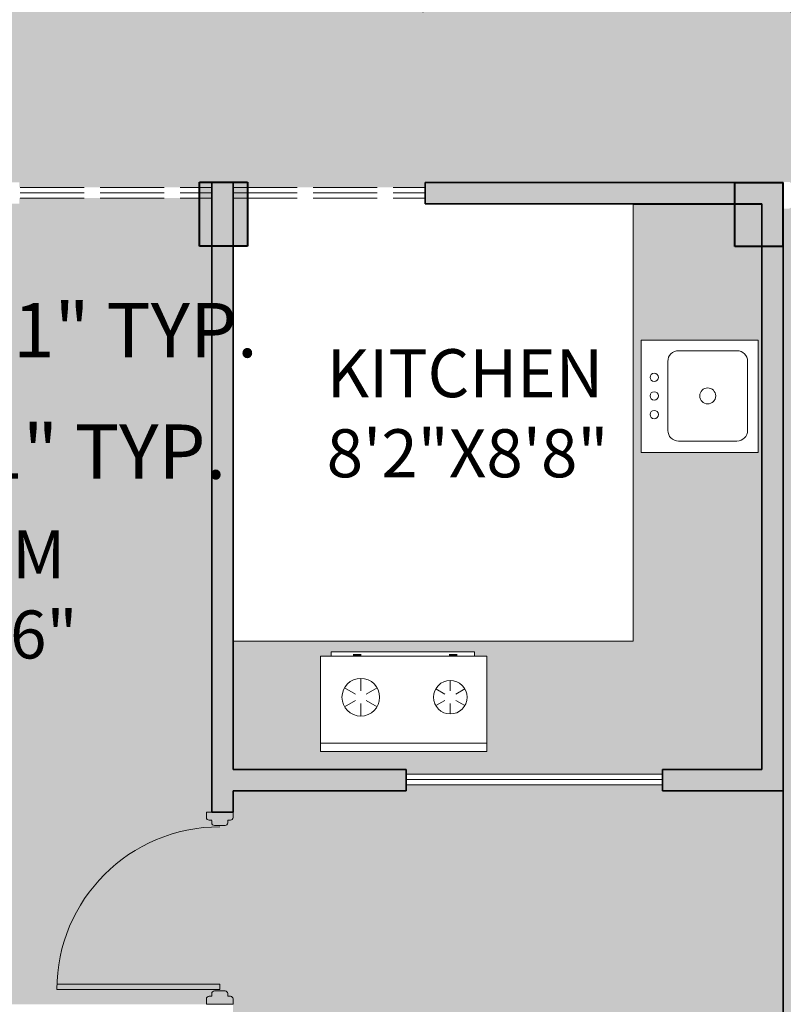
# Model space of a CAD drawing. Units: inches. Extents: x 1077 to 2505, y 1892 to 2728.
# Tile 5 of 26: x 1290 to 1433, y 2153 to 2338. Entities that reach past the tile are written whole.
import ezdxf

# ---------------------------------------------------------------- set-up
doc = ezdxf.new("R2010")
doc.units = ezdxf.units.IN
doc.linetypes.add('ACAD_ISO02W100', pattern=[15, 12, -3])
doc.layers.get('Defpoints').update_dxf_attribs({"color": 220, "linetype": 'ACAD_ISO02W100'})
for name, color, linetype, lineweight in [('00 FURNITURE', 15, 'Continuous', 15), ('A-ANNO-DIMS', 2, 'Continuous', 18), ('A-AREA-IDEN', 7, 'Continuous', 18), ('A-COLS', 7, 'Continuous', 40), ('A-DOOR', 4, 'Continuous', 18), ('A-EQPM', 8, 'Continuous', 13), ('A-FLOR-CASE', 8, 'Continuous', 18), ('A-FLOR-FIXT', 8, 'Continuous', 13), ('A-GLAZ-OVHD', 160, 'ACAD_ISO02W100', 13), ('A_TEXT_SMALL', 18, 'Continuous', 13), ('WALL', 7, 'Continuous', 35), ('WINDOW', 160, 'Continuous', 13)]:
    doc.layers.add(name, color=color, linetype=linetype, lineweight=lineweight)
doc.layers.add('A-FLOR-PATT', color=254, linetype='Continuous', lineweight=9, true_color=0xd7ebd2)
doc.layers.add('FURN3D', color=229, linetype='Continuous', lineweight=5, true_color=0x4a3f41)
doc.styles.get("Standard").update_dxf_attribs({"font": 'arial.ttf'})
doc.dimstyles.get("Standard").update_dxf_attribs({"dimtxt": 10.18, "dimasz": 0.18, "dimexe": 0.18, "dimexo": 0.0625, "dimgap": 0.09, "dimtad": 0, "dimtih": 1, "dimtoh": 1, "dimdec": 0, "dimzin": 0, "dimdsep": 46, "dimlunit": 3, "dimtxsty": 'Standard', "dimcen": 0.09, "dimadec": 0, "dimazin": 0, "dimtfac": 1, "dimtdec": 0, "dimtofl": 0, "dimtmove": 0, "dimatfit": 3, "dimfxl": 1, "dimtolj": 1, "dimtzin": 0, "dimarcsym": 0})

# ---------------------------------------------------------------- blocks, each defined once
blk = doc.blocks.new('DDD')
at = {"layer": '00 FURNITURE'}
for p, q in [((-12579.77, -15859.53), (-12579.77, -15829.05)), ((-12578.77, -15859.53), (-12578.77, -15829.03)), ((-12612.02, -15857.03), (-12612.02, -15862.03)), ((-12611.02, -15857.03), (-12612.02, -15857.03)), ((-12610.52, -15858.03), (-12610.52, -15857.53)), ((-12577.52, -15858.03), (-12577.52, -15857.53)), ((-12577.02, -15857.03), (-12576.02, -15857.03)), ((-12576.02, -15857.03), (-12576.02, -15862.03)), ((-12578.77, -15859.53), (-12579.77, -15859.53)), ((-12610.52, -15861.53), (-12610.52, -15861.03)), ((-12577.52, -15861.53), (-12577.52, -15861.03)), ((-12612.02, -15862.03), (-12611.02, -15862.03)), ((-12576.02, -15862.03), (-12577.02, -15862.03))]:
    blk.add_line(p, q, dxfattribs=at)
for points in [[(-12610.52, -15861.03), (-12610.02, -15861.03, 0.414214), (-12609.52, -15860.53), (-12609.52, -15858.53, 0.414214), (-12610.02, -15858.03), (-12610.52, -15858.03)], [(-12577.52, -15861.03), (-12578.02, -15861.03, -0.414214), (-12578.52, -15860.53), (-12578.52, -15858.53, -0.414214), (-12578.02, -15858.03), (-12577.52, -15858.03)]]:
    blk.add_lwpolyline(points, format="xyb", dxfattribs=at)
for centre, radius, start, end in [((-12578.77, -15859.53), 30.5, 90, 180), ((-12611.02, -15857.53), 0.5, 0, 90), ((-12577.02, -15857.53), 0.5, 90, 180), ((-12611.02, -15861.53), 0.5, 270, 0), ((-12577.02, -15861.53), 0.5, 180, 270)]:
    blk.add_arc(centre, radius, start, end, dxfattribs=at)
blk = doc.blocks.new('A$C21540130')
at = {"layer": 'FURN3D'}
for p, q in [((1.57, 0), (1.57, 31.11)), ((9.61, 25.31), (8.63, 27.01)), ((10.79, 25.31), (11.77, 27.01)), ((9.02, 24.29, -27.54), (7.06, 24.29, -27.54)), ((11.38, 24.29, -27.54), (13.34, 24.29, -27.54)), ((9.61, 23.27), (8.63, 21.57)), ((10.79, 23.27), (11.77, 21.57)), ((9.61, 8.56), (8.43, 10.6)), ((10.79, 8.56), (11.97, 10.6)), ((9.02, 7.54), (6.67, 7.54)), ((11.38, 7.54), (13.73, 7.54)), ((9.61, 6.52), (8.43, 4.48)), ((10.79, 6.52), (11.97, 4.48))]:
    blk.add_line(p, q, dxfattribs=at)
for points in [[(0, 0), (0, 31.11), (17.9, 31.11), (17.9, 0)], [(18.68, 1.96), (18.68, 28.83), (17.9, 28.83), (17.9, 1.96)]]:
    blk.add_lwpolyline(points, close=True, dxfattribs=at)
for centre, radius in [((10.2, 24.29), 3.14), ((10.2, 7.54), 3.53)]:
    blk.add_circle(centre, radius, dxfattribs=at)
for points in [[(17.9, 24.03), (18.29, 24.03), (17.9, 25.6), (18.29, 25.6)], [(17.9, 6.05), (18.29, 6.05), (17.9, 7.62), (18.29, 7.62)]]:
    blk.add_solid(points, dxfattribs=at)
blk = doc.blocks.new('reh-flat-2')
at = {"layer": 'A_TEXT_SMALL'}
for p, q in [((486053827.2, -394630231.2), (486054182.4, -394629799.8)), ((486054182.4, -394629799.8), (486054596.6, -394630140.9)), ((486054228.6, -394629903.6), (486054483.5, -394630113.5)), ((486053979.5, -394630126.3), (486054157.1, -394629910.6)), ((486054596.6, -394630140.9), (486054241.4, -394630572.3)), ((486054490.4, -394630185), (486054312.8, -394630400.7)), ((486054241.4, -394630572.3), (486053827.2, -394630231.2)), ((486054241.3, -394630407.7), (486053986.4, -394630197.8))]:
    blk.add_line(p, q, dxfattribs=at)
for centre, radius in [((486054234.9, -394630155.7), 38.1), ((486054004.1, -394630296.2), 20.1), ((486054072.7, -394630352.7), 20.1), ((486054141.4, -394630409.3), 20.1)]:
    blk.add_circle(centre, radius, dxfattribs=at)
for centre, start, end in [((486054196.3, -394629942.9), 50.5305, 140.5305), ((486054018.7, -394630158.5), 140.5305, 230.5305), ((486054451.2, -394630152.8), 320.5305, 50.5305), ((486054273.6, -394630368.4), 230.5305, 320.5305)]:
    blk.add_arc(centre, 50.8, start, end, dxfattribs=at)
blk = doc.blocks.new('C1')
h = blk.add_hatch(color=256)
h.dxf.hatch_style = 1
h.paths.add_polyline_path([(1668.56, 2445.41), (1677.56, 2445.41), (1677.56, 2457.41), (1668.56, 2457.41)])
for p, q in [((1668.56, 2457.41), (1677.56, 2457.41)), ((1668.56, 2445.41), (1668.56, 2457.41)), ((1677.56, 2457.41), (1677.56, 2445.41)), ((1677.56, 2445.41), (1668.56, 2445.41))]:
    blk.add_line(p, q)
blk = doc.blocks.new('WINDOW-48-PARTITION')
for p, q in [((48, 2), (0, 2)), ((48, 1), (0, 1)), ((48, 0), (0, 0))]:
    blk.add_line(p, q)
blk = doc.blocks.new('*D36')
at = {"layer": 'A-ANNO-DIMS', "color": 0, "lineweight": -2, "transparency": 16777216}
for p, q in [((1365.09, 2349.48), (1365.09, 2339.05)), ((1433.87, 2349.48), (1433.87, 2339.05)), ((1365.27, 2339.23), (1433.69, 2339.23)), ((1433.87, 2339.23), (1434.05, 2339.23))]:
    blk.add_line(p, q, dxfattribs=at)
at = {"layer": 'A-ANNO-DIMS', "color": 0, "transparency": 16777216}
for points in [[(1365.27, 2339.26), (1365.27, 2339.2), (1365.09, 2339.23)], [(1433.69, 2339.26), (1433.69, 2339.2), (1433.87, 2339.23)]]:
    blk.add_solid(points, dxfattribs=at)
at = {"layer": 'Defpoints', "color": 0, "transparency": 16777216}
for p in [(1365.09, 2349.54), (1433.87, 2349.54), (1433.87, 2339.23)]:
    blk.add_point(p, dxfattribs=at)
at = {"layer": 'A-ANNO-DIMS', "color": 0, "transparency": 16777216, "insert": (1507.58, 2339.23), "char_height": 10.18, "attachment_point": 5}
blk.add_mtext('\\A1;DINING SET 5\'-9" TYP.', dxfattribs=at)
blk = doc.blocks.new('*D38')
at = {"layer": 'A-ANNO-DIMS', "color": 0, "lineweight": -2, "transparency": 16777216}
for p, q in [((1258.04, 2297.01), (1263.41, 2297.01)), ((1263.23, 2296.83), (1263.23, 2284.84)), ((1263.23, 2262.15), (1263.23, 2274.13)), ((1258.04, 2261.97), (1263.41, 2261.97))]:
    blk.add_line(p, q, dxfattribs=at)
at = {"layer": 'A-ANNO-DIMS', "color": 0, "transparency": 16777216}
for points in [[(1263.2, 2296.83), (1263.26, 2296.83), (1263.23, 2297.01)], [(1263.2, 2262.15), (1263.26, 2262.15), (1263.23, 2261.97)]]:
    blk.add_solid(points, dxfattribs=at)
at = {"layer": 'Defpoints', "color": 0, "transparency": 16777216}
for p in [(1257.98, 2297.01), (1263.23, 2297.01), (1257.98, 2261.97)]:
    blk.add_point(p, dxfattribs=at)
at = {"layer": 'A-ANNO-DIMS', "color": 0, "transparency": 16777216, "insert": (1263.23, 2279.49), "char_height": 10.18, "attachment_point": 5}
blk.add_mtext('\\A1;ARMCHAIR 2\'-11" TYP.', dxfattribs=at)
blk = doc.blocks.new('*D39')
at = {"layer": 'A-ANNO-DIMS', "color": 0, "lineweight": -2, "transparency": 16777216}
for p, q in [((1222.94, 2261.91), (1222.94, 2256.53)), ((1257.98, 2261.91), (1257.98, 2256.53)), ((1223.12, 2256.71), (1257.8, 2256.71)), ((1257.98, 2256.71), (1258.16, 2256.71))]:
    blk.add_line(p, q, dxfattribs=at)
at = {"layer": 'A-ANNO-DIMS', "color": 0, "transparency": 16777216}
for points in [[(1223.12, 2256.74), (1223.12, 2256.68), (1222.94, 2256.71)], [(1257.8, 2256.74), (1257.8, 2256.68), (1257.98, 2256.71)]]:
    blk.add_solid(points, dxfattribs=at)
at = {"layer": 'Defpoints', "color": 0, "transparency": 16777216}
for p in [(1222.94, 2261.97), (1257.98, 2261.97), (1257.98, 2256.71)]:
    blk.add_point(p, dxfattribs=at)
at = {"layer": 'A-ANNO-DIMS', "color": 0, "transparency": 16777216, "insert": (1293.31, 2256.71), "char_height": 10.18, "attachment_point": 5}
blk.add_mtext('\\A1;2\'-11" TYP.', dxfattribs=at)

msp = doc.modelspace()

# ---------------------------------------------------------------- hatches: boundary and pattern name
at = {"layer": 'A-FLOR-PATT', "transparency": 33554559}
h = msp.add_hatch(color=256, dxfattribs=at)
h.dxf.hatch_style = 1
h.paths.add_polyline_path([(1395.53, 2577.16), (1374.83, 2577.16), (1350.83, 2577.19), (1350.83, 2577.16), (1329.53, 2577.16), (1329.53, 2480.16), (1329.53, 2469.16), (1325.53, 2469.16), (1325.53, 2515.13), (1307.53, 2515.13), (1307.53, 2577.16), (1269.31, 2577.16), (1221.31, 2577.15), (1221.31, 2577.16), (1187.53, 2577.16), (1187.53, 2433.16), (1289.53, 2433.16), (1289.53, 2429.16), (1263.53, 2429.16), (1187.53, 2429.16), (1187.53, 2395.02), (1187.53, 2395.02), (1187.53, 2371.02), (1187.53, 2371.02), (1187.53, 2307.16), (1259.53, 2307.16), (1259.53, 2399.16), (1263.53, 2399.16), (1263.53, 2307.16), (1289.53, 2307.16), (1289.53, 2306.23), (1325.53, 2306.23), (1325.53, 2307.16), (1329.53, 2307.16), (1329.53, 2306.23), (1365.53, 2306.23), (1365.53, 2307.16), (1432.53, 2307.16), (1432.53, 2088.16), (1547.53, 2088.16), (1547.53, 2140.08), (1511.53, 2140.08), (1511.53, 2267.16), (1475.53, 2267.16), (1475.53, 2303.16), (1468.53, 2303.16), (1468.53, 2307.16), (1547.53, 2307.16), (1547.53, 2348.22), (1547.53, 2396.22), (1547.53, 2429.16), (1435.53, 2429.16), (1435.53, 2433.16), (1476.35, 2433.16), (1476.35, 2451.18), (1547.53, 2451.18), (1547.53, 2577.16), (1499.53, 2577.16), (1499.53, 2586.16), (1547.53, 2586.16), (1547.53, 2642.16), (1518.18, 2642.16), (1518.18, 2642.05), (1494.15, 2642.05), (1494.15, 2642.16), (1469.53, 2642.16), (1469.53, 2577.16), (1399.53, 2577.16), (1399.53, 2429.16), (1325.53, 2429.16), (1325.53, 2433.16), (1329.53, 2433.16), (1395.53, 2433.16), (1395.53, 2480.16), (1359.53, 2480.16), (1359.53, 2484.16), (1395.53, 2484.16)])
h.paths.add_polyline_path([(1357.65, 2482.07), (1355.65, 2482.07), (1355.65, 2481.07, 0.414214), (1356.65, 2480.07), (1344.65, 2480.07), (1344.65, 2477.06), (1343.27, 2477.06), (1343.27, 2480.07), (1330.65, 2480.07, -0.414214), (1329.65, 2481.07), (1329.65, 2484.07), (1331.65, 2484.07), (1331.65, 2510.07, -0.446908)], flags=16)
h.paths.add_polyline_path([(1305.09, 2559.18), (1288.89, 2559.18), (1288.89, 2575.38), (1305.09, 2575.38)], flags=16)
h.paths.add_polyline_path([(1304.19, 2560.08), (1289.79, 2560.08), (1289.79, 2574.48), (1304.19, 2574.48)], flags=0)
h.paths.add_polyline_path([(1287.99, 2500.68, -0.414214), (1287.09, 2499.78), (1265.14, 2499.78), (1224.09, 2499.78, -0.414214), (1223.19, 2500.68), (1223.19, 2557.16), (1223.19, 2571.74), (1223.19, 2575.38), (1287.99, 2575.38), (1287.99, 2571.74), (1287.09, 2571.74, -0.414214), (1287.99, 2570.84)], flags=16)
h.paths.add_polyline_path([(1292.98, 2569.05, -1), (1300.92, 2569.05, -1)], flags=0)
h.paths.add_polyline_path([(1293.32, 2569.05, -1), (1300.58, 2569.05, -1)], flags=0)
h.paths.add_polyline_path([(1322.8, 2462.21), (1322.8, 2431.71), (1323.05, 2430.71), (1323.05, 2431.71), (1321.8, 2431.71), (1321.8, 2462.19, 0.404641), (1292.3, 2431.71), (1292.05, 2430.71, -0.414214), (1291.55, 2430.21), (1291.05, 2430.21), (1291.05, 2429.71, -0.414214), (1290.55, 2429.21), (1289.55, 2429.21), (1289.55, 2434.21), (1290.55, 2434.21, -0.414214), (1291.05, 2433.71), (1291.05, 2433.21), (1291.55, 2433.21, -0.414214), (1292.05, 2432.71), (1292.3, 2431.71, -0.414214)], flags=16)
h.paths.add_polyline_path([(1287.82, 2548.28, 0.292232), (1279.17, 2536.8, 0.052719), (1223.93, 2548.28), (1223.28, 2548.28), (1223.28, 2557.16), (1223.93, 2557.16), (1245.42, 2557.16, -0.117785), (1245.77, 2557.93, -0.059418), (1254.87, 2567.02, -0.379859), (1257.28, 2566.88, -0.02509), (1261.41, 2563.32, -0.025935), (1265.65, 2567.02, -0.379859), (1268.06, 2566.88, -0.061767), (1277.52, 2557.43, -0.069393), (1277.82, 2557.16), (1287.82, 2557.16)], flags=0)
h.paths.add_polyline_path([(1263.47, 2548.28), (1260.56, 2548.28, -0.015371), (1258.01, 2546.13, -0.429576), (1255.37, 2546.06, -0.016036), (1252.69, 2548.28), (1223.28, 2548.28), (1223.28, 2554.42), (1246.78, 2554.42, 0.055344), (1255.37, 2546.06, 0.331768), (1257.52, 2545.74, 0.027343), (1262, 2549.64, 0.00919)], flags=0)
h.paths.add_polyline_path([(1295.56, 2568.34), (1296.87, 2569.09), (1296.87, 2570.6, 0.399698), (1295.39, 2569.05, 0.119004)], flags=0)
h.paths.add_polyline_path([(1295.21, 2569.05, -1), (1298.68, 2569.05, -1)], flags=0)
h.paths.add_polyline_path([(1296.95, 2568.96), (1297.03, 2569), (1297.03, 2569.09), (1296.99, 2569.11), (1296.91, 2568.98)], flags=0)
h.paths.add_polyline_path([(1402.28, 2462.19, -0.414214), (1432.78, 2431.69), (1433.03, 2432.69), (1432.78, 2431.69, 0.404641), (1403.28, 2462.17), (1403.28, 2431.69), (1402.03, 2431.69), (1402.03, 2430.69, -0.414214), (1401.53, 2430.19), (1401.03, 2430.19), (1401.03, 2429.69, -0.414214), (1400.53, 2429.19), (1399.53, 2429.19), (1399.53, 2434.19), (1400.53, 2434.19, -0.414214), (1401.03, 2433.69), (1401.03, 2433.19), (1401.53, 2433.19, -0.414214), (1402.03, 2432.69)], flags=16)
h.paths.add_polyline_path([(1470.16, 2535.21, -0.414214), (1471.06, 2536.11), (1527.54, 2536.11), (1542.12, 2536.11), (1545.76, 2536.11), (1545.76, 2471.31), (1542.12, 2471.31), (1542.12, 2472.21, -0.414214), (1541.22, 2471.31), (1471.06, 2471.31, -0.414214), (1470.16, 2472.21), (1470.16, 2494.16)], flags=16)
h.paths.add_polyline_path([(1483.07, 2536.11, 0.253465), (1480.11, 2526.15, 0.2538), (1470.15, 2523.19)], flags=16)
h.paths.add_polyline_path([(1223.19, 2512.69, 0.253465), (1233.14, 2509.74, 0.2538), (1236.1, 2499.77)], flags=16)
h.paths.add_polyline_path([(1469.77, 2578.72), (1469.77, 2581.72), (1471.77, 2581.72), (1471.77, 2607.72, -0.01951), (1473.77, 2607.68), (1473.77, 2579.72), (1473.77, 2578.72, -0.414214), (1472.77, 2577.72), (1470.77, 2577.72, -0.414214)], flags=16)
h.paths.add_polyline_path([(1382.46, 2398.13), (1395.04, 2398.13), (1395.04, 2399.74), (1382.46, 2399.74)], flags=16)
h.paths.add_polyline_path([(1379.94, 2397.18), (1379.94, 2389.82), (1380.5, 2389.82), (1380.5, 2396.05, -0.41429), (1381.06, 2396.61), (1396.47, 2396.61, -0.414213), (1397.03, 2396.05), (1397.03, 2389.82), (1397.59, 2389.82), (1397.59, 2397.18)], flags=16)
h.paths.add_polyline_path([(1263.37, 2428.14), (1263.37, 2426.14, -0.414214), (1262.37, 2425.14), (1261.37, 2425.14), (1233.41, 2425.14, 0.400854), (1259.37, 2401.04), (1259.37, 2401.14), (1261.37, 2401.14, -0.446908), (1233.37, 2427.14), (1259.37, 2427.14), (1259.37, 2429.14), (1262.37, 2429.14, -0.414214)], flags=16)
h.paths.add_polyline_path([(1404.79, 2398.13), (1417.37, 2398.13), (1417.37, 2399.74), (1404.79, 2399.74)], flags=16)
h.paths.add_polyline_path([(1402.27, 2397.18), (1404.79, 2398.13), (1417.37, 2398.13), (1419.92, 2397.18)], flags=16)
h.paths.add_polyline_path([(1432.26, 2383.16), (1432.26, 2370.59), (1433.87, 2370.59), (1433.87, 2383.16)], flags=16)
h.paths.add_polyline_path([(1431.3, 2385.69), (1423.84, 2385.69), (1423.84, 2385.13), (1430.18, 2385.13, -0.41429), (1430.74, 2384.57), (1430.74, 2369.16, -0.414237), (1430.18, 2368.6), (1423.84, 2368.6), (1423.84, 2368.03), (1431.3, 2368.03)], flags=16)
h.paths.add_polyline_path([(1417.37, 2351.16), (1417.37, 2349.54), (1418.9, 2349.54, 0.414236), (1419.92, 2350.56), (1419.92, 2352.11)], flags=16)
h.paths.add_polyline_path([(1395.04, 2351.16), (1395.04, 2349.54), (1396.58, 2349.54, 0.414235), (1397.59, 2350.56), (1397.59, 2352.11)], flags=16)
h.paths.add_polyline_path([(1366.7, 2370.05), (1365.09, 2370.05), (1365.09, 2368.52, 0.414235), (1366.11, 2367.5), (1367.66, 2367.5)], flags=16)
h.paths.add_polyline_path([(1419.36, 2359.47), (1419.36, 2353.24, -0.41419), (1418.8, 2352.68), (1403.39, 2352.68, -0.414137), (1402.83, 2353.24), (1402.83, 2359.47), (1397.03, 2359.47), (1397.03, 2353.24, -0.414189), (1396.47, 2352.68), (1381.06, 2352.68, -0.414137), (1380.5, 2353.24), (1380.5, 2359.47)], flags=16)
h.paths.add_polyline_path([(1222.29, 2559.18), (1206.09, 2559.18), (1206.09, 2575.38), (1222.29, 2575.38)], flags=16)
h.paths.add_polyline_path([(1221.39, 2560.08), (1206.99, 2560.08), (1206.99, 2574.48), (1221.39, 2574.48)], flags=0)
h.paths.add_polyline_path([(1482, 2577.72), (1482, 2580.73), (1483.38, 2580.73), (1483.38, 2577.72), (1484.77, 2577.72), (1484.77, 2574.72), (1483.38, 2574.72), (1483.38, 2577.72)], flags=16)
h.paths.add_polyline_path([(1266.37, 2415.53), (1266.37, 2414.14), (1263.37, 2414.14), (1263.37, 2415.53), (1260.36, 2415.53), (1260.36, 2416.91), (1263.37, 2416.91), (1263.37, 2415.53)], flags=16)
h.paths.add_polyline_path([(1210.26, 2569.05, -1), (1218.19, 2569.05, -1)], flags=0)
h.paths.add_polyline_path([(1210.6, 2569.05, -1), (1217.85, 2569.05, -1)], flags=0)
h.paths.add_polyline_path([(1212.84, 2568.34), (1214.15, 2569.09), (1214.15, 2570.6, 0.399698), (1212.67, 2569.05, 0.119004)], flags=0)
h.paths.add_polyline_path([(1212.49, 2569.05, -1), (1215.96, 2569.05, -1)], flags=0)
h.paths.add_polyline_path([(1214.23, 2568.96), (1214.3, 2568.91), (1214.3, 2569)], flags=0)
h.paths.add_polyline_path([(1507.18, 2480.12, 0.052719), (1518.66, 2535.36), (1518.66, 2536.01), (1527.54, 2536.01), (1527.54, 2535.36), (1527.54, 2513.88, -0.117785), (1528.31, 2513.53, -0.059418), (1537.4, 2504.43, -0.379859), (1537.26, 2502.01, -0.02509), (1533.7, 2497.89, -0.025935), (1537.4, 2493.64, -0.379859), (1537.26, 2491.23, -0.061767), (1527.8, 2481.77, -0.069393), (1527.54, 2481.47), (1527.54, 2471.47), (1518.66, 2471.47, 0.292232)], flags=0)
h.paths.add_polyline_path([(1516.43, 2503.92, -0.016036), (1518.66, 2506.6), (1518.66, 2536.01), (1524.8, 2536.01), (1524.8, 2512.51, 0.055344), (1516.43, 2503.92, 0.331768), (1516.12, 2501.77, 0.027343), (1520.01, 2497.29, 0.00919), (1518.66, 2495.82), (1518.66, 2498.73, -0.015371), (1516.5, 2501.28, -0.429576)], flags=0)
h.paths.add_polyline_path([(1499.63, 2625.5, -0.171636), (1502.82, 2631.01), (1502.82, 2633.37), (1498.68, 2633.37, -0.414214), (1497.7, 2634.36), (1497.7, 2640.66, -0.414214), (1498.68, 2641.64), (1514.82, 2641.64, -0.414214), (1515.81, 2640.66), (1515.81, 2634.36, -0.414214), (1514.82, 2633.37), (1510.69, 2633.37), (1510.69, 2631.01, -0.171636), (1513.88, 2625.5, -0.258205), (1509.31, 2614.47), (1504.19, 2614.47, -0.258205)], flags=16)
h.paths.add_polyline_path([(1501.2, 2625.5, -0.171636), (1504.39, 2631.01), (1509.12, 2631.01, -0.171636), (1512.3, 2625.5, -0.210384), (1509.35, 2616.02), (1504.16, 2616.02, -0.210384)], flags=0)
h.paths.add_polyline_path([(1529.56, 2537.01), (1529.56, 2553.21), (1545.76, 2553.21), (1545.76, 2537.01)], flags=16)
h.paths.add_polyline_path([(1530.46, 2537.91), (1530.46, 2552.31), (1544.86, 2552.31), (1544.86, 2537.91)], flags=0)
h.paths.add_polyline_path([(1535.45, 2545.07, -1), (1543.39, 2545.07, -1)], flags=0)
h.paths.add_polyline_path([(1535.8, 2545.07, -1), (1543.05, 2545.07, -1)], flags=0)
h.paths.add_polyline_path([(1529.56, 2470.41), (1545.76, 2470.41), (1545.76, 2454.21), (1529.56, 2454.21)], flags=16)
h.paths.add_polyline_path([(1541.16, 2544.99), (1540.98, 2544.99, -0.544606), (1538.71, 2543.68), (1538.62, 2543.53, 0.547962)], flags=0)
h.paths.add_polyline_path([(1530.46, 2469.51), (1544.86, 2469.51), (1544.86, 2455.11), (1530.46, 2455.11)], flags=0)
h.paths.add_polyline_path([(1539.47, 2545.14), (1539.42, 2545.22), (1539.38, 2545.14)], flags=0)
h.paths.add_polyline_path([(1543.39, 2462.34, -1), (1535.45, 2462.34, -1)], flags=0)
h.paths.add_polyline_path([(1543.05, 2462.34, -1), (1535.8, 2462.34, -1)], flags=0)
h.paths.add_polyline_path([(1541.16, 2462.27), (1540.98, 2462.27, -0.544606), (1538.71, 2460.96), (1538.62, 2460.8, 0.547962)], flags=0)
h.paths.add_polyline_path([(1539.47, 2462.42), (1539.42, 2462.5), (1539.38, 2462.42)], flags=0)
h.paths.add_polyline_path([(1435.32, 2335.25, -0.414214), (1465.82, 2304.75), (1466.07, 2305.75), (1465.82, 2304.75, 0.404641), (1436.32, 2335.23), (1436.32, 2304.75), (1435.07, 2304.75), (1435.07, 2303.75, -0.414214), (1434.57, 2303.25), (1434.07, 2303.25), (1434.07, 2302.75, -0.414214), (1433.57, 2302.25), (1432.57, 2302.25), (1432.57, 2307.25), (1433.57, 2307.25, -0.414214), (1434.07, 2306.75), (1434.07, 2306.25), (1434.57, 2306.25, -0.414214), (1435.07, 2305.75)], flags=16)
h.paths.add_polyline_path([(1532.13, 2635.71), (1535.43, 2635.71), (1535.43, 2635.89), (1532.13, 2635.89)], flags=16)
edge = h.paths.add_edge_path(flags=16)
edge.add_arc((1535.98, 2632.67), 0.183, 270, 360)
edge.add_line((1536.17, 2632.67), (1536.17, 2639.82))
edge.add_line((1536.17, 2639.82), (1538.29, 2639.82))
edge.add_line((1538.29, 2639.82), (1538.29, 2641.82))
edge.add_line((1538.29, 2641.82), (1533.25, 2641.82))
edge.add_line((1533.25, 2641.82), (1533.25, 2639.82))
edge.add_line((1533.25, 2639.82), (1534.87, 2639.82))
edge.add_line((1534.87, 2639.82), (1534.87, 2639))
edge.add_line((1534.87, 2639), (1533.7, 2639))
edge.add_line((1533.7, 2639), (1533.7, 2639.82))
edge.add_line((1533.7, 2639.82), (1533.25, 2639.82))
edge.add_line((1533.25, 2639.82), (1533.25, 2641.82))
edge.add_line((1533.25, 2641.82), (1538.29, 2641.82))
edge.add_line((1538.29, 2641.82), (1538.29, 2641.34))
edge.add_line((1538.29, 2641.34), (1540.64, 2641.58))
edge.add_line((1540.64, 2641.58), (1540.64, 2641.82))
edge.add_line((1540.64, 2641.82), (1541.5, 2641.82))
edge.add_line((1541.5, 2641.82), (1541.5, 2641.25))
edge.add_line((1541.5, 2641.25), (1541.31, 2639.79))
edge.add_ellipse((1541.09, 2638.95), major_axis=(-1.08, 0), ratio=0.790849, start_angle=180, end_angle=255.2976, ccw=False)
edge.add_line((1542.17, 2638.95), (1542.17, 2638.38))
edge.add_ellipse((1541.09, 2638.38), major_axis=(-1.08, 0), ratio=0.790849, start_angle=0, end_angle=180, ccw=False)
edge.add_line((1540, 2638.38), (1540.01, 2638.87))
edge.add_ellipse((1541.09, 2638.95), major_axis=(-1.08, 0), ratio=0.790849, start_angle=284.7024, end_angle=364.0401, ccw=False)
edge.add_line((1540.78, 2639.75), (1540.78, 2641.25))
edge.add_line((1540.78, 2641.25), (1540.64, 2641.25))
edge.add_line((1540.64, 2641.25), (1538.29, 2641.01))
edge.add_line((1538.29, 2641.01), (1538.29, 2639.82))
edge.add_line((1538.29, 2639.82), (1536.17, 2639.82))
edge.add_line((1536.17, 2639.82), (1536.17, 2632.48))
edge.add_line((1536.17, 2632.48), (1535.98, 2632.48))
h.paths.add_polyline_path([(1496.32, 2250.34, -0.292371), (1498.9, 2247.83, -0.085148), (1501.21, 2208.85, -0.01331), (1500.27, 2098.5, -0.379287), (1497.22, 2095.28, -0.0502), (1441.54, 2095.28, -0.379287), (1438.5, 2098.5, -0.01331), (1437.56, 2208.85, -0.086132), (1439.96, 2248.26, -0.295116), (1442.59, 2250.78, -0.114238)], flags=16)
h.paths.add_polyline_path([(1495.16, 2205.84, -0.355389), (1496.7, 2202.1), (1492.94, 2189.65, -0.398275), (1489.12, 2187.47, 0.113332), (1449.64, 2187.47, -0.398275), (1445.82, 2189.65), (1442.06, 2202.1, -0.355394), (1443.6, 2205.84, -0.265725)], flags=0)
h.paths.add_polyline_path([(1440.37, 2195.72), (1445.94, 2181.67), (1445.94, 2160.63), (1440.84, 2157.26)], flags=0)
h.paths.add_polyline_path([(1498.46, 2195.72), (1497.99, 2157.26), (1492.88, 2160.63), (1492.88, 2181.67)], flags=0)
h.paths.add_polyline_path([(1445.94, 2158.37), (1445.94, 2137.12), (1441.12, 2122.56), (1440.87, 2155.03)], flags=0)
h.paths.add_polyline_path([(1492.88, 2158.37), (1497.96, 2155.03), (1497.71, 2122.56), (1492.88, 2137.12)], flags=0)
h.paths.add_polyline_path([(1489.88, 2130.4), (1494.39, 2107.67, -0.090102), (1444.44, 2107.65), (1448.95, 2130.39, 0.036636)], flags=0)
h.paths.add_polyline_path([(1447.54, 2159.34), (1497.44, 2159.34), (1497.44, 2177.89), (1447.54, 2177.89)], flags=8)
h.paths.add_polyline_path([(1196.44, 2354.84), (1246.65, 2354.84), (1246.65, 2388.43), (1196.44, 2388.43)], flags=24)
h.paths.add_polyline_path([(1296.09, 2360.25), (1353.81, 2360.25), (1353.81, 2393.84), (1296.09, 2393.84)], flags=24)
h.paths.add_polyline_path([(1400.72, 2471.85), (1470.63, 2471.85), (1470.63, 2505.44), (1400.72, 2505.44)], flags=24)
h.paths.add_polyline_path([(1324.78, 2448.48), (1394.95, 2448.48), (1394.95, 2467.02), (1324.78, 2467.02)], flags=24)
h.paths.add_polyline_path([(1335.08, 2531.43), (1389.67, 2531.43), (1389.67, 2565.02), (1335.08, 2565.02)], flags=24)
h.paths.add_polyline_path([(1225.76, 2460), (1295.67, 2460), (1295.67, 2493.58), (1225.76, 2493.58)], flags=24)
h = msp.add_hatch(color=256, dxfattribs=at)
h.dxf.hatch_style = 1
h.paths.add_polyline_path([(1547.53, 2348.22), (1547.53, 2396.22), (1547.53, 2425.11), (1547.53, 2425.11), (1547.53, 2429.16), (1435.53, 2429.16), (1434.03, 2429.21), (1434.03, 2430.19), (1433.03, 2430.19), (1432.78, 2431.69, 0.404641), (1403.28, 2462.17), (1403.28, 2431.69), (1402.03, 2431.69), (1402.03, 2430.19), (1401.03, 2430.19), (1401.03, 2429.19), (1399.53, 2429.19), (1399.53, 2429.19), (1399.53, 2429.16), (1334.67, 2429.16), (1334.67, 2423.95), (1325.67, 2423.95), (1325.67, 2429.16), (1325.53, 2429.16), (1324.05, 2429.24), (1324.05, 2430.21), (1323.05, 2430.21), (1323.05, 2431.71), (1321.8, 2431.71), (1321.8, 2462.19, 0.416544), (1292.05, 2430.73, -0.423614), (1291.55, 2430.21), (1291.05, 2430.21), (1291.05, 2429.21), (1289.55, 2429.21), (1289.53, 2429.21), (1289.53, 2429.16), (1263.37, 2429.16), (1263.37, 2415.53), (1266.37, 2415.53), (1266.37, 2414.14), (1263.37, 2414.14), (1263.37, 2399.16), (1263.53, 2399.16), (1263.53, 2307.16), (1289.53, 2307.16), (1289.53, 2306.23), (1323.26, 2306.23), (1323.26, 2307.21), (1332.26, 2307.21), (1365.53, 2306.23), (1365.53, 2307.16), (1432.53, 2307.16), (1432.57, 2307.16), (1432.57, 2307.25), (1434.07, 2307.25), (1434.07, 2306.25), (1435.32, 2306.25), (1435.32, 2335.25, -0.407346), (1466.07, 2305.73, -0.423614), (1466.57, 2306.25), (1467.07, 2306.25), (1467.07, 2307.25), (1468.57, 2307.25), (1547.53, 2307.16), (1547.53, 2307.2)])
h.paths.add_polyline_path([(1430.74, 2369.16), (1430.74, 2384.57, 0.41429), (1430.18, 2385.13), (1423.84, 2385.13), (1423.84, 2368.6), (1430.18, 2368.6, 0.414237)], flags=16)
h.paths.add_polyline_path([(1432.26, 2383.16), (1432.26, 2370.59), (1433.87, 2370.59), (1433.87, 2383.16)], flags=16)
h.paths.add_polyline_path([(1431.3, 2368.03), (1431.3, 2385.69), (1432.26, 2383.16), (1432.26, 2370.59)], flags=16)
h.paths.add_polyline_path([(1417.37, 2351.16), (1417.37, 2349.54), (1418.9, 2349.54, 0.414236), (1419.92, 2350.56), (1419.92, 2352.11)], flags=16)
h.paths.add_polyline_path([(1403.39, 2352.68), (1418.78, 2352.68, 0.42427), (1419.36, 2353.24), (1419.36, 2359.47), (1402.83, 2359.47), (1402.83, 2353.24, 0.414137)], flags=16)
h.paths.add_polyline_path([(1366.7, 2370.05), (1365.09, 2370.05), (1365.09, 2368.52, 0.414235), (1366.11, 2367.5), (1367.66, 2367.5)], flags=16)
h.paths.add_polyline_path([(1382.46, 2398.13), (1395.04, 2398.13), (1395.04, 2399.74), (1382.46, 2399.74)], flags=16)
h.paths.add_polyline_path([(1396.47, 2396.61), (1381.06, 2396.61, 0.41429), (1380.5, 2396.05), (1380.5, 2389.82), (1397.03, 2389.82), (1397.03, 2396.05, 0.414213)], flags=16)
h.paths.add_polyline_path([(1402.27, 2397.18), (1402.83, 2396.05, -0.414213), (1403.39, 2396.61)], flags=16)
h.paths.add_polyline_path([(1418.8, 2396.61), (1419.36, 2396.61), (1419.36, 2396.05, 0.414237)], flags=16)
h.paths.add_polyline_path([(1404.79, 2398.13), (1417.37, 2398.13), (1417.37, 2399.74), (1404.79, 2399.74)], flags=16)
h.paths.add_polyline_path([(1381.06, 2352.68, -0.414213), (1380.5, 2353.24), (1380.27, 2352.11)], flags=16)
h.paths.add_polyline_path([(1396.58, 2349.54), (1396.58, 2349.54), (1395.04, 2349.54), (1395.04, 2349.54), (1382.46, 2349.54), (1382.46, 2351.16), (1395.04, 2351.16), (1397.59, 2352.11), (1397.59, 2350.56, -0.414235)], flags=16)
h.paths.add_polyline_path([(1379.94, 2397.18), (1382.46, 2398.13), (1395.04, 2398.13), (1397.59, 2397.18)], flags=16)
h.paths.add_polyline_path([(1368.78, 2384.59, 0.414213), (1368.22, 2384.03), (1367.66, 2367.5), (1367.66, 2385.15)], flags=16)
h.paths.add_polyline_path([(1547.53, 2574.38), (1547.51, 2574.38), (1547.51, 2577.16), (1499.53, 2577.16), (1484.77, 2577.44), (1484.77, 2574.72), (1483.38, 2574.72), (1483.38, 2577.72), (1482, 2577.72), (1469.53, 2577.72), (1469.53, 2577.16), (1401.95, 2577.16), (1401.95, 2574.12), (1399.53, 2574.12), (1399.53, 2434.19), (1401.03, 2434.19), (1401.03, 2433.19), (1402.28, 2433.19), (1402.28, 2462.19, -0.407346), (1433.03, 2432.67, -0.423614), (1433.53, 2433.19), (1434.03, 2433.19), (1434.03, 2434.19), (1435.53, 2434.19), (1476.35, 2433.81), (1476.35, 2451.18), (1547.53, 2451.18)])
h.paths.add_polyline_path([(1470.16, 2535.21, -0.414214), (1471.06, 2536.11), (1527.54, 2536.11), (1542.12, 2536.11), (1545.76, 2536.11), (1545.76, 2471.31), (1542.12, 2471.31), (1542.12, 2472.21, -0.414214), (1541.22, 2471.31), (1471.06, 2471.31, -0.414214), (1470.16, 2472.21), (1470.16, 2494.16)], flags=16)
h.paths.add_polyline_path([(1483.07, 2536.11, 0.253465), (1480.11, 2526.15, 0.2538), (1470.15, 2523.19)], flags=16)
h.paths.add_polyline_path([(1525.55, 2481.52, -0.000893), (1524.8, 2482.24), (1524.8, 2471.47), (1527.54, 2471.47), (1527.54, 2472.12), (1527.54, 2481.47, -0.388819)], flags=0)
h.paths.add_polyline_path([(1518.66, 2536.01), (1527.54, 2536.01), (1527.54, 2535.36), (1527.54, 2513.88, -0.117785), (1528.31, 2513.53, -0.059418), (1537.4, 2504.43, -0.379859), (1537.26, 2502.01, -0.02509), (1533.7, 2497.89, 0.033431), (1528.3, 2502.74, 0.308459), (1526.25, 2502.88, 0.047827), (1518.66, 2495.82), (1518.66, 2498.73, -0.015371), (1516.5, 2501.28, -0.429576), (1516.43, 2503.92, -0.016036), (1518.66, 2506.6)], flags=0)
h.paths.add_polyline_path([(1529.56, 2537.01), (1529.56, 2553.21), (1545.76, 2553.21), (1545.76, 2537.01)], flags=16)
h.paths.add_polyline_path([(1530.46, 2537.91), (1530.46, 2552.31), (1544.86, 2552.31), (1544.86, 2537.91)], flags=0)
h.paths.add_polyline_path([(1535.8, 2545.07, -1), (1543.05, 2545.07, -1)], flags=0)
h.paths.add_polyline_path([(1541.16, 2544.99), (1540.98, 2544.99, -0.544606), (1538.71, 2543.68), (1538.62, 2543.53, 0.547962)], flags=0)
h.paths.add_polyline_path([(1539.47, 2545.14), (1539.42, 2545.22), (1539.38, 2545.14)], flags=0)
h.paths.add_polyline_path([(1529.56, 2470.41), (1545.76, 2470.41), (1545.76, 2454.21), (1529.56, 2454.21)], flags=16)
h.paths.add_polyline_path([(1530.46, 2469.51), (1544.86, 2469.51), (1544.86, 2455.11), (1530.46, 2455.11)], flags=0)
h.paths.add_polyline_path([(1535.8, 2462.34, -1), (1543.05, 2462.34, -1)], flags=0)
h.paths.add_polyline_path([(1541.16, 2462.27), (1540.98, 2462.27, -0.544606), (1538.71, 2460.96), (1538.62, 2460.8, 0.547962)], flags=0)
h.paths.add_polyline_path([(1539.47, 2462.42), (1539.42, 2462.5), (1539.38, 2462.42)], flags=0)
h.paths.add_polyline_path([(1395.53, 2574.12), (1392.95, 2574.12), (1392.95, 2577.16), (1374.83, 2577.16), (1350.83, 2577.19), (1350.83, 2577.16), (1332.07, 2577.16), (1332.07, 2574), (1329.53, 2574), (1329.53, 2484.07), (1331.65, 2484.07), (1331.65, 2510.07, -0.423677), (1357.76, 2484.07), (1359.53, 2484.07), (1359.53, 2484.16), (1395.53, 2484.16)], flags=17)
h.paths.add_polyline_path([(1395.53, 2480.16), (1359.06, 2480.16, 0.437533), (1359.53, 2481.55), (1359.53, 2484.16), (1395.53, 2484.16), (1395.53, 2574.12), (1392.95, 2574.12), (1392.95, 2577.16), (1374.83, 2577.16), (1350.83, 2577.19), (1350.83, 2577.16), (1332.07, 2577.16), (1332.07, 2574), (1329.53, 2574), (1329.53, 2484.07), (1329.65, 2484.07), (1329.65, 2481.07), (1329.53, 2480.16), (1329.53, 2469.16), (1325.53, 2469.16), (1325.53, 2515.13), (1307.53, 2515.13), (1307.53, 2577.16), (1269.31, 2577.16), (1221.31, 2577.15), (1221.31, 2577.16), (1187.61, 2577.16), (1187.61, 2574.03), (1187.53, 2433.16), (1289.55, 2433.16), (1289.55, 2434.21), (1291.05, 2434.21), (1291.05, 2433.21), (1292.05, 2433.21), (1292.3, 2431.71, -0.414214), (1322.8, 2462.21), (1323.05, 2432.71, -0.414214), (1323.55, 2433.21), (1324.05, 2433.21), (1324.05, 2434.21), (1325.67, 2434.21), (1325.67, 2435.95), (1334.67, 2435.95), (1334.67, 2433.16), (1395.53, 2433.16)])
h.paths.add_polyline_path([(1344.65, 2480.07), (1344.65, 2477.06), (1343.27, 2477.06), (1343.27, 2480.07), (1332.65, 2480.07, 0.414214), (1333.65, 2481.07), (1333.65, 2482.07), (1331.65, 2482.07), (1331.65, 2484.07), (1331.65, 2510.07, -0.446908), (1357.65, 2482.07), (1355.65, 2482.07), (1355.65, 2481.07, 0.414214), (1356.65, 2480.07)], flags=16)
h.paths.add_polyline_path([(1287.99, 2500.68, -0.414214), (1287.09, 2499.78), (1265.14, 2499.78), (1224.09, 2499.78, -0.414214), (1223.19, 2500.68), (1223.19, 2557.16), (1223.19, 2571.74), (1223.19, 2575.38), (1287.99, 2575.38), (1287.99, 2571.74), (1287.09, 2571.74, -0.414214), (1287.99, 2570.84)], flags=16)
h.paths.add_polyline_path([(1277.77, 2555.17, -0.000893), (1277.05, 2554.42), (1287.82, 2554.42), (1287.82, 2557.16), (1287.17, 2557.16), (1277.82, 2557.16, -0.388819)], flags=0)
h.paths.add_polyline_path([(1223.28, 2548.28), (1223.28, 2557.16), (1223.93, 2557.16), (1245.42, 2557.16, -0.117785), (1245.77, 2557.93, -0.059418), (1254.87, 2567.02, -0.379859), (1257.28, 2566.88, -0.02509), (1261.41, 2563.32, 0.033431), (1256.55, 2557.93, 0.308459), (1256.41, 2555.88, 0.047827), (1263.47, 2548.28), (1260.56, 2548.28, -0.015371), (1258.01, 2546.13, -0.429576), (1255.37, 2546.06, -0.016036), (1252.69, 2548.28)], flags=0)
h.paths.add_polyline_path([(1305.09, 2559.18), (1288.89, 2559.18), (1288.89, 2575.38), (1305.09, 2575.38)], flags=16)
h.paths.add_polyline_path([(1304.19, 2560.08), (1289.79, 2560.08), (1289.79, 2574.48), (1304.19, 2574.48)], flags=0)
h.paths.add_polyline_path([(1300.58, 2569.05, -1), (1293.32, 2569.05, -1)], flags=0)
h.paths.add_polyline_path([(1223.19, 2512.69, 0.253465), (1233.14, 2509.74, 0.2538), (1236.1, 2499.77)], flags=16)
h.paths.add_polyline_path([(1295.56, 2568.34), (1296.87, 2569.09), (1296.87, 2570.6, 0.399698), (1295.39, 2569.05, 0.119004)], flags=0)
h.paths.add_polyline_path([(1295.21, 2569.05, -1), (1298.68, 2569.05, -1)], flags=0)
h.paths.add_polyline_path([(1296.95, 2568.96), (1297.03, 2569), (1297.03, 2569.09), (1296.99, 2569.11), (1296.91, 2568.98)], flags=0)
h.paths.add_polyline_path([(1222.29, 2559.18), (1206.09, 2559.18), (1206.09, 2575.38), (1222.29, 2575.38)], flags=16)
h.paths.add_polyline_path([(1221.39, 2560.08), (1206.99, 2560.08), (1206.99, 2574.48), (1221.39, 2574.48)], flags=0)
h.paths.add_polyline_path([(1217.85, 2569.05, -1), (1210.6, 2569.05, -1)], flags=0)
h.paths.add_polyline_path([(1212.84, 2568.34), (1214.15, 2569.09), (1214.15, 2570.6, 0.399698), (1212.67, 2569.05, 0.119004)], flags=0)
h.paths.add_polyline_path([(1212.49, 2569.05, -1), (1215.96, 2569.05, -1)], flags=0)
h.paths.add_polyline_path([(1214.23, 2568.96), (1214.3, 2569), (1214.3, 2569.09), (1214.26, 2569.11), (1214.19, 2568.98)], flags=0)
h.paths.add_polyline_path([(1259.53, 2399.14), (1259.37, 2399.14), (1259.37, 2401.04, -0.423677), (1233.37, 2427.14), (1259.37, 2427.14), (1259.37, 2429.16), (1187.53, 2429.16), (1187.53, 2395.02), (1187.53, 2395.02), (1187.53, 2371.02), (1187.53, 2371.02), (1187.53, 2311.49), (1187.55, 2311.49), (1187.55, 2307.16), (1259.53, 2307.16)])
h.paths.add_polyline_path([(1323.26, 2295.21), (1323.26, 2304.23), (1289.53, 2304.23), (1289.53, 2303.16), (1187.55, 2303.16), (1187.55, 2299.49), (1178.53, 2299.49), (1178.53, 2267.66), (1178.53, 2219.66), (1182.03, 2219.66), (1182.03, 2267.67), (1184.03, 2267.67), (1184.03, 2219.66), (1187.53, 2219.66), (1187.53, 2153.16), (1228.13, 2153.16), (1276.13, 2153.16), (1276.13, 2153.16), (1324.54, 2153.16), (1324.54, 2154.67), (1325.54, 2154.67), (1325.54, 2155.92), (1296.54, 2155.92, -0.407346), (1326.06, 2186.67, -0.423614), (1325.54, 2187.17), (1325.54, 2187.67), (1324.54, 2187.67), (1324.54, 2189.17), (1325.43, 2295.21)])
h.paths.add_polyline_path([(1432.53, 2307.16), (1365.53, 2307.16), (1365.53, 2306.23), (1365.53, 2303.16), (1428.53, 2303.16), (1428.53, 2221.2), (1428.57, 2221.2), (1428.57, 2197.2), (1428.53, 2197.16), (1428.53, 2303.01), (1404.46, 2303.01), (1404.46, 2221.2), (1329.53, 2221.2), (1329.53, 2307.16), (1325.53, 2307.16), (1325.53, 2295.21), (1325.43, 2295.21), (1324.54, 2189.17), (1324.54, 2187.67), (1326.04, 2187.67, 1.016365), (1326.06, 2186.67, 0.407348), (1296.54, 2155.92), (1325.54, 2155.92), (1325.54, 2154.67), (1324.54, 2154.67), (1324.54, 2153.16), (1329.53, 2153.16), (1329.53, 2144.16), (1432.53, 2144.16)])
h.paths.add_polyline_path([(1361.95, 2194.26), (1361.95, 2193.16), (1329.53, 2193.16), (1329.53, 2189.16), (1329.54, 2188.17), (1329.54, 2189.16), (1329.53, 2189.16), (1329.53, 2193.16), (1361.95, 2193.16), (1361.95, 2196.26), (1409.95, 2196.26), (1409.95, 2194.26)], flags=16)
h.paths.add_polyline_path([(1377.02, 2200.5), (1345.91, 2200.5), (1345.91, 2218.4), (1347.87, 2218.4), (1347.87, 2219.18), (1374.75, 2219.18), (1374.75, 2218.4), (1377.02, 2218.4)], flags=16)
h.paths.add_polyline_path([(1367.07, 2210.7, -1), (1373.34, 2210.7, -1)], flags=0)
h.paths.add_polyline_path([(1349.92, 2210.7, -1), (1356.98, 2210.7, -1)], flags=0)
h.paths.add_polyline_path([(1405.95, 2256.57), (1405.95, 2277.6), (1427.86, 2277.6), (1427.86, 2256.57)], flags=16)
h.paths.add_polyline_path([(1412.92, 2258.68, -0.414201), (1410.93, 2260.67), (1410.93, 2273.62, -0.414239), (1412.92, 2275.61), (1423.88, 2275.61, -0.414227), (1425.87, 2273.62), (1425.87, 2260.67, -0.414214), (1423.88, 2258.68)], flags=0)
h.paths.add_polyline_path([(1407.61, 2263.66, -1), (1409.18, 2263.66, -1)], flags=0)
h.paths.add_polyline_path([(1407.61, 2267.14, -1), (1409.18, 2267.14, -1)], flags=0)
h.paths.add_polyline_path([(1416.91, 2267.15, -1), (1419.89, 2267.15, -1)], flags=0)
h.paths.add_polyline_path([(1407.61, 2270.63, -1), (1409.18, 2270.63, -1)], flags=0)
h.paths.add_polyline_path([(1475.53, 2303.16), (1468.57, 2303.16), (1468.57, 2302.25), (1467.07, 2302.25), (1467.07, 2303.25), (1466.07, 2303.25), (1465.82, 2304.75, 0.404641), (1436.32, 2335.23), (1436.32, 2304.75), (1435.07, 2304.75), (1435.07, 2303.25), (1434.07, 2303.25), (1434.07, 2302.25), (1432.53, 2302.25), (1432.53, 2144.16), (1432.53, 2088.16), (1547.52, 2088.16), (1547.52, 2100.19), (1547.52, 2140.08), (1511.53, 2140.08), (1511.53, 2267.16), (1475.53, 2267.16)])
h.paths.add_polyline_path([(1438.35, 2102.86, 0.033498), (1438.37, 2102.21, -0.000079)], flags=16)
h.paths.add_polyline_path([(1496.32, 2250.34, -0.292371), (1498.9, 2247.83, -0.085148), (1501.21, 2208.85, -0.012784), (1500.42, 2102.86, -0.033498), (1500.39, 2102.21, 0.012863), (1501.21, 2208.85, 0.077283), (1499.67, 2244.3, 0.265882), (1497.48, 2246.8, 0.14401), (1441.46, 2247.36, 0.270646), (1439.21, 2244.85, -0.007564), (1439.96, 2248.26, -0.295116), (1442.59, 2250.78, -0.114238)], flags=16)
h.paths.add_polyline_path([(1495.16, 2205.84, -0.355389), (1496.7, 2202.1), (1492.94, 2189.65, -0.398275), (1489.12, 2187.47, 0.113332), (1449.64, 2187.47, -0.398275), (1445.82, 2189.65), (1442.06, 2202.1, -0.355394), (1443.6, 2205.84, -0.265725)], flags=16)
h.paths.add_polyline_path([(1440.37, 2195.72), (1445.94, 2181.67), (1445.94, 2160.63), (1440.84, 2157.26)], flags=16)
h.paths.add_polyline_path([(1498.46, 2195.72), (1497.99, 2157.26), (1492.88, 2160.63), (1492.88, 2181.67)], flags=16)
h.paths.add_polyline_path([(1445.94, 2158.37), (1445.94, 2137.12), (1441.12, 2122.56), (1440.87, 2155.03)], flags=16)
h.paths.add_polyline_path([(1492.88, 2158.37), (1497.96, 2155.03), (1497.71, 2122.56), (1492.88, 2137.12)], flags=16)
h.paths.add_polyline_path([(1489.88, 2130.4), (1494.39, 2107.67, -0.090102), (1444.44, 2107.65), (1448.95, 2130.39, 0.036636)], flags=16)
h.paths.add_polyline_path([(1296.09, 2360.25), (1353.81, 2360.25), (1353.81, 2393.84), (1296.09, 2393.84)], flags=24)
h.paths.add_polyline_path([(1400.72, 2471.85), (1470.63, 2471.85), (1470.63, 2505.44), (1400.72, 2505.44)], flags=24)
h.paths.add_polyline_path([(1335.08, 2531.43), (1389.67, 2531.43), (1389.67, 2565.02), (1335.08, 2565.02)], flags=24)
h.paths.add_polyline_path([(1324.78, 2448.48), (1394.95, 2448.48), (1394.95, 2467.02), (1324.78, 2467.02)], flags=24)
h.paths.add_polyline_path([(1225.76, 2460), (1295.67, 2460), (1295.67, 2493.58), (1225.76, 2493.58)], flags=24)
h.paths.add_polyline_path([(1196.44, 2354.84), (1246.65, 2354.84), (1246.65, 2388.43), (1196.44, 2388.43)], flags=24)
h.paths.add_polyline_path([(1447.54, 2159.34), (1497.44, 2159.34), (1497.44, 2177.89), (1447.54, 2177.89)], flags=24)

# ---------------------------------------------------------------- linework, layer by layer
at = {"layer": 'A-FLOR-CASE'}
for p, q in [((1428.46, 2303.01), (1404.46, 2303.01)), ((1404.46, 2303.01), (1404.46, 2221.2)), ((1404.46, 2221.2), (1329.53, 2221.2)), ((1428.57, 2221.2), (1428.53, 2221.2)), ((1428.57, 2197.2), (1428.57, 2221.2))]:
    msp.add_line(p, q, dxfattribs=at)
at = {"layer": 'A-GLAZ-OVHD'}
for p, q in [((1289.65, 2306.23), (1325.53, 2306.23)), ((1329.53, 2306.23), (1365.53, 2306.23)), ((1289.65, 2305.23), (1325.53, 2305.23)), ((1289.65, 2304.23), (1325.53, 2304.23)), ((1329.53, 2305.23), (1365.53, 2305.23)), ((1329.53, 2304.23), (1365.53, 2304.23))]:
    msp.add_line(p, q, dxfattribs=at)
at = {"layer": 'WALL'}
for p, q in [((1325.53, 2189.16), (1325.53, 2307.16)), ((1325.53, 2307.16), (1329.53, 2307.16)), ((1329.53, 2197.16), (1329.53, 2307.16)), ((1365.53, 2303.16), (1365.53, 2307.16)), ((1365.53, 2307.16), (1432.53, 2307.16)), ((1432.53, 2088.16), (1432.53, 2307.16)), ((1365.53, 2303.16), (1428.53, 2303.16)), ((1428.53, 2197.16), (1428.53, 2303.16)), ((1329.53, 2197.16), (1361.95, 2197.16)), ((1361.95, 2193.16), (1361.95, 2197.16)), ((1409.95, 2193.16), (1409.95, 2197.16)), ((1409.95, 2197.16), (1428.53, 2197.16)), ((1329.53, 2189.16), (1329.53, 2193.16)), ((1329.53, 2193.16), (1361.95, 2193.16)), ((1409.95, 2193.16), (1432.53, 2193.16)), ((1325.53, 2189.16), (1329.53, 2189.16))]:
    msp.add_line(p, q, dxfattribs=at)

# ---------------------------------------------------------------- block references
at = {"layer": 'A-COLS'}
for p in [(-345.3, -150.2), (-245.08, -150.27)]:
    msp.add_blockref('C1', p, dxfattribs=at)
at = {"layer": 'A-DOOR', "xscale": -1, "rotation": 90}
msp.add_blockref('DDD', (-14532.49, -10422.85), dxfattribs=at)
at = {"layer": 'A-EQPM', "xscale": -1, "rotation": 270}
msp.add_blockref('A$C21540130', (1345.91, 2200.5), dxfattribs=at)
at = {"layer": 'A-FLOR-FIXT', "xscale": 0.0391972730482577, "yscale": 0.0391972730482577, "zscale": 0.0391972730482577, "rotation": 309.4694759622496}
msp.add_blockref('reh-flat-2', (-168252.82, 24542481.88), dxfattribs=at)
at = {"layer": 'WINDOW'}
msp.add_blockref('WINDOW-48-PARTITION', (1361.99, 2194.26), dxfattribs=at)

# ---------------------------------------------------------------- texts
at = {"layer": 'A-AREA-IDEN', "char_height": 9, "attachment_point": 1}
for s, insert in [('KITCHEN\\P8\'2"X8\'8"', (1347.06, 2275.91)), ('\\pxi-3,l4,t4;DRG.ROOM\\P10\'6"X12\'6"', (1225.03, 2241.96))]:
    msp.add_mtext_dynamic_manual_height_columns(s, width=128.1076, gutter_width=12.5, heights=[0], dxfattribs=dict(at, insert=insert))

# ---------------------------------------------------------------- dimensions: what is measured, and where the dimension line sits
at = {"layer": 'A-ANNO-DIMS'}
for base, p1, p2, text, picture, middle in [((1433.87, 2339.23), (1365.09, 2349.54), (1433.87, 2349.54), 'DINING SET <> TYP.', '*D36', (1507.58, 2339.23)), ((1257.98, 2256.71), (1222.94, 2261.97), (1257.98, 2261.97), '<> TYP.', '*D39', (1293.31, 2256.71))]:
    dim = msp.add_linear_dim(base=base, p1=p1, p2=p2, text=text, dimstyle='Standard', override={"dimdec": 1, "dimlfac": 1, "dimrnd": 0, "dimzin": 1, "dimdsep": 46, "dimlunit": 4, "dimfrac": 2}, dxfattribs=at)
    dim.commit()
    dim.dimension.update_dxf_attribs({"geometry": picture, "text_midpoint": middle})
dim = msp.add_linear_dim(base=(1263.23, 2297.01), p1=(1257.98, 2261.97), p2=(1257.98, 2297.01), angle=90, text='ARMCHAIR <> TYP.', dimstyle='Standard', override={"dimdec": 1, "dimlfac": 1, "dimrnd": 0, "dimzin": 1, "dimdsep": 46, "dimlunit": 4, "dimfrac": 2}, dxfattribs=at)
dim.commit()
dim.dimension.update_dxf_attribs({"geometry": '*D38', "text_midpoint": (1263.23, 2279.49)})

doc.saveas('drawing.dxf')
